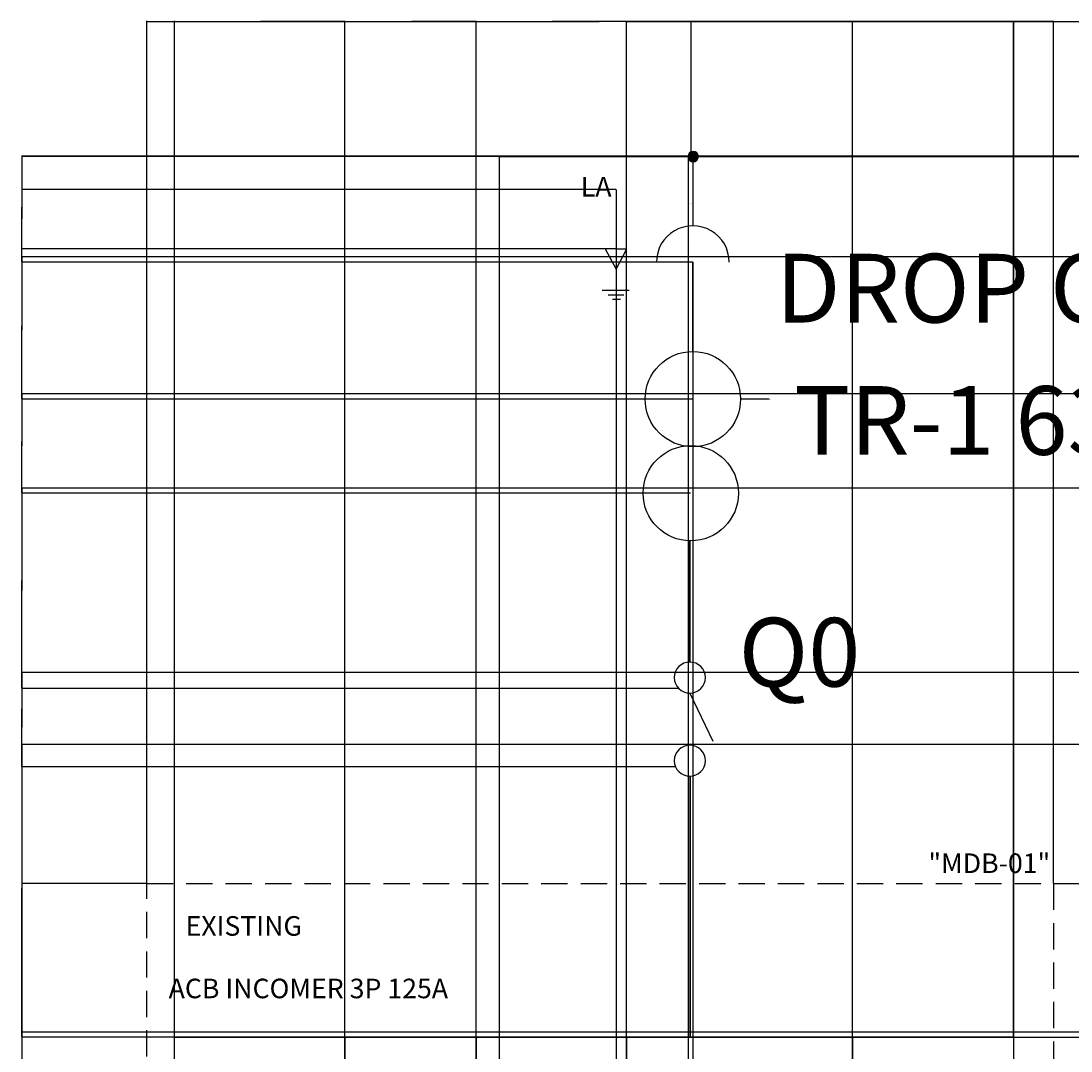
# Model space of a CAD drawing. Units: millimetres. Extents: x 1832 to 3146, y 927 to 1751.
# Tile 2 of 4: x 1832 to 2339, y 1253 to 1751. Entities that reach past the tile are written whole.
import ezdxf

# ---------------------------------------------------------------- set-up
doc = ezdxf.new("R2010")
doc.units = ezdxf.units.MM
doc.header["$MEASUREMENT"] = 0
doc.linetypes.add('DASHED', pattern=[19.05, 12.7, -6.35])
doc.layers.get('0').update_dxf_attribs({"color": 2, "lineweight": 35})
doc.layers.get('0').transparency = 0.01
for name, color, linetype, lineweight in [('A-ANNO-DIMS', 2, 'Continuous', 18), ('E-ANNO-TEXT', 7, 'Continuous', 18), ('E-POWR-EQPM', 2, 'Continuous', 25), ('E-POWR-PNLS', 3, 'DASHED', 25), ('E-POWR-WIRE', 7, 'Continuous', 35)]:
    doc.layers.add(name, color=color, linetype=linetype, lineweight=lineweight)
doc.styles.get("Standard").update_dxf_attribs({"font": 'arial.ttf'})
doc.dimstyles.get("Standard").update_dxf_attribs({"dimtxt": 0.18, "dimasz": 0.18, "dimexe": 0.18, "dimexo": 0.0625, "dimgap": 0.09, "dimtad": 0, "dimtih": 1, "dimtoh": 1, "dimdec": 4, "dimzin": 0, "dimdsep": 46, "dimtxsty": 'Standard', "dimcen": 0.09, "dimadec": 0, "dimazin": 0, "dimtfac": 1, "dimtdec": 4, "dimtofl": 0, "dimtmove": 0, "dimatfit": 3, "dimfxl": 1, "dimtolj": 1, "dimtzin": 0, "dimarcsym": 0})

# ---------------------------------------------------------------- blocks, each defined once
blk = doc.blocks.new('CB-INCOMER')
blk.add_line((2155.16, 1426.14), (2166.26, 1402.88))
for points in [[(2147.67, 1433.64, 1), (2162.67, 1433.64, 1)], [(2147.67, 1393.5, 1), (2162.67, 1393.5, 1)]]:
    blk.add_lwpolyline(points, format="xyb", close=True)
blk = doc.blocks.new('LIGHTNING-ARRESTER')
for p, q in [((2119.54, 1669.38), (2119.54, 1640.82)), ((2119.54, 1640.82), (2114.27, 1640.82)), ((2114.27, 1640.82), (2119.54, 1630.9)), ((2119.54, 1640.82), (2124.8, 1640.82)), ((2119.54, 1630.9), (2124.8, 1640.82)), ((2119.54, 1630.9), (2119.54, 1620.77)), ((2112.86, 1620.77), (2125.9, 1620.77)), ((2115.79, 1618.51), (2123.28, 1618.51)), ((2117.89, 1616.41), (2121.66, 1616.41))]:
    blk.add_line(p, q)
blk = doc.blocks.new('DROPOUT-FUSE')
h = blk.add_hatch(color=256)
h.dxf.hatch_style = 1
h.paths.add_polyline_path([(2154.3, 1685.32), (2159.3, 1685.32, 1)])
h.paths.add_polyline_path([(2159.3, 1685.32), (2154.3, 1685.32, 1)])
blk.add_line((2156.63, 1682.82), (2156.63, 1651.9))
blk.add_lwpolyline([(2154.3, 1685.32, 1), (2159.3, 1685.32, 1)], format="xyb", close=True)
blk.add_arc((2156.63, 1634.33), 17.57, 359.971, 180.029)
blk = doc.blocks.new('TRANSFORMER')
for centre in [(2156.63, 1568.17), (2155.63, 1522.72)]:
    blk.add_circle(centre, 23.01)
blk = doc.blocks.new('*D11')
at = {"layer": 'A-ANNO-DIMS', "color": 0, "lineweight": -2, "transparency": 16777216}
for p, q in [((1892.88, 1334.1), (1832.41, 1334.1)), ((1832.59, 1333.92), (1832.59, 1168.69)), ((1832.59, 1003.11), (1832.59, 1168.33)), ((1892.88, 1002.93), (1832.41, 1002.93))]:
    blk.add_line(p, q, dxfattribs=at)
at = {"layer": 'A-ANNO-DIMS', "color": 0, "lineweight": 35, "transparency": 16777216}
for points in [[(1832.56, 1333.92), (1832.62, 1333.92), (1832.59, 1334.1)], [(1832.56, 1003.11), (1832.62, 1003.11), (1832.59, 1002.93)]]:
    blk.add_solid(points, dxfattribs=at)
at = {"layer": 'Defpoints', "color": 0, "lineweight": 35, "transparency": 16777216}
for p in [(1832.59, 1334.1), (1892.94, 1334.1), (1892.94, 1002.93)]:
    blk.add_point(p, dxfattribs=at)
at = {"layer": 'A-ANNO-DIMS', "color": 0, "transparency": 16777216, "insert": (1832.59, 1168.51), "char_height": 0.18, "attachment_point": 5}
blk.add_mtext('\\A1;331.2', dxfattribs=at)
blk = doc.blocks.new('*D12')
at = {"layer": 'A-ANNO-DIMS', "color": 0, "lineweight": -2, "transparency": 16777216}
for p, q in [((1906.41, 1259.94), (1906.41, 1750.84)), ((1906.59, 1750.66), (1947.09, 1750.66)), ((1988.37, 1750.66), (1947.87, 1750.66)), ((1988.55, 1259.94), (1988.55, 1750.84))]:
    blk.add_line(p, q, dxfattribs=at)
at = {"layer": 'A-ANNO-DIMS', "color": 0, "lineweight": 35, "transparency": 16777216}
for points in [[(1906.59, 1750.69), (1906.59, 1750.63), (1906.41, 1750.66)], [(1988.37, 1750.69), (1988.37, 1750.63), (1988.55, 1750.66)]]:
    blk.add_solid(points, dxfattribs=at)
at = {"layer": 'Defpoints', "color": 0, "lineweight": 35, "transparency": 16777216}
for p in [(1988.55, 1750.66), (1906.41, 1259.88), (1988.55, 1259.88)]:
    blk.add_point(p, dxfattribs=at)
at = {"layer": 'A-ANNO-DIMS', "color": 0, "transparency": 16777216, "insert": (1947.48, 1750.66), "char_height": 0.18, "attachment_point": 5}
blk.add_mtext('\\A1;82.14', dxfattribs=at)
blk = doc.blocks.new('*D13')
at = {"layer": 'A-ANNO-DIMS', "color": 0, "lineweight": -2, "transparency": 16777216}
for p, q in [((1988.55, 1259.94), (1988.55, 1750.84)), ((1988.73, 1750.66), (2019.92, 1750.66)), ((2051.9, 1750.66), (2020.71, 1750.66)), ((2052.08, 1259.94), (2052.08, 1750.84))]:
    blk.add_line(p, q, dxfattribs=at)
at = {"layer": 'A-ANNO-DIMS', "color": 0, "lineweight": 35, "transparency": 16777216}
for points in [[(1988.73, 1750.69), (1988.73, 1750.63), (1988.55, 1750.66)], [(2051.9, 1750.69), (2051.9, 1750.63), (2052.08, 1750.66)]]:
    blk.add_solid(points, dxfattribs=at)
at = {"layer": 'Defpoints', "color": 0, "lineweight": 35, "transparency": 16777216}
for p in [(2052.08, 1750.66), (1988.55, 1259.88), (2052.08, 1259.88)]:
    blk.add_point(p, dxfattribs=at)
at = {"layer": 'A-ANNO-DIMS', "color": 0, "transparency": 16777216, "insert": (2020.31, 1750.66), "char_height": 0.18, "attachment_point": 5}
blk.add_mtext('\\A1;63.53', dxfattribs=at)
blk = doc.blocks.new('*D14')
at = {"layer": 'A-ANNO-DIMS', "color": 0, "lineweight": -2, "transparency": 16777216}
for p, q in [((2052.08, 1259.94), (2052.08, 1750.84)), ((2052.26, 1750.66), (2087.91, 1750.66)), ((2124.35, 1750.66), (2088.7, 1750.66)), ((2124.53, 1259.94), (2124.53, 1750.84))]:
    blk.add_line(p, q, dxfattribs=at)
at = {"layer": 'A-ANNO-DIMS', "color": 0, "lineweight": 35, "transparency": 16777216}
for points in [[(2052.26, 1750.69), (2052.26, 1750.63), (2052.08, 1750.66)], [(2124.35, 1750.69), (2124.35, 1750.63), (2124.53, 1750.66)]]:
    blk.add_solid(points, dxfattribs=at)
at = {"layer": 'Defpoints', "color": 0, "lineweight": 35, "transparency": 16777216}
for p in [(2124.53, 1750.66), (2052.08, 1259.88), (2124.53, 1259.88)]:
    blk.add_point(p, dxfattribs=at)
at = {"layer": 'A-ANNO-DIMS', "color": 0, "transparency": 16777216, "insert": (2088.31, 1750.66), "char_height": 0.18, "attachment_point": 5}
blk.add_mtext('\\A1;72.45', dxfattribs=at)
blk = doc.blocks.new('*D15')
at = {"layer": 'A-ANNO-DIMS', "color": 0, "lineweight": -2, "transparency": 16777216}
for p, q in [((2124.53, 1259.94), (2124.53, 1750.84)), ((2124.71, 1750.66), (2178.71, 1750.66)), ((2233.62, 1750.66), (2179.62, 1750.66)), ((2233.8, 1259.94), (2233.8, 1750.84))]:
    blk.add_line(p, q, dxfattribs=at)
at = {"layer": 'A-ANNO-DIMS', "color": 0, "lineweight": 35, "transparency": 16777216}
for points in [[(2124.71, 1750.69), (2124.71, 1750.63), (2124.53, 1750.66)], [(2233.62, 1750.69), (2233.62, 1750.63), (2233.8, 1750.66)]]:
    blk.add_solid(points, dxfattribs=at)
at = {"layer": 'Defpoints', "color": 0, "lineweight": 35, "transparency": 16777216}
for p in [(2233.8, 1750.66), (2124.53, 1259.88), (2233.8, 1259.88)]:
    blk.add_point(p, dxfattribs=at)
at = {"layer": 'A-ANNO-DIMS', "color": 0, "transparency": 16777216, "insert": (2179.17, 1750.66), "char_height": 0.18, "attachment_point": 5}
blk.add_mtext('\\A1;109.27', dxfattribs=at)
blk = doc.blocks.new('*D21')
at = {"layer": 'A-ANNO-DIMS', "color": 0, "lineweight": -2, "transparency": 16777216}
for p, q in [((2155.83, 1687.68), (2155.83, 1750.84)), ((2156.01, 1750.66), (2407.13, 1750.66)), ((2659.03, 1750.66), (2407.91, 1750.66)), ((2659.21, 1690.18), (2659.21, 1750.84))]:
    blk.add_line(p, q, dxfattribs=at)
at = {"layer": 'A-ANNO-DIMS', "color": 0, "lineweight": 35, "transparency": 16777216}
for points in [[(2156.01, 1750.69), (2156.01, 1750.63), (2155.83, 1750.66)], [(2659.03, 1750.69), (2659.03, 1750.63), (2659.21, 1750.66)]]:
    blk.add_solid(points, dxfattribs=at)
at = {"layer": 'Defpoints', "color": 0, "lineweight": 35, "transparency": 16777216}
for p in [(2659.21, 1750.66), (2659.21, 1690.11), (2155.83, 1687.62)]:
    blk.add_point(p, dxfattribs=at)
at = {"layer": 'A-ANNO-DIMS', "color": 0, "transparency": 16777216, "insert": (2407.52, 1750.66), "char_height": 0.18, "attachment_point": 5}
blk.add_mtext('\\A1;503.4', dxfattribs=at)
blk = doc.blocks.new('*D23')
at = {"layer": 'A-ANNO-DIMS', "color": 0, "lineweight": -2, "transparency": 16777216}
for p, q in [((2156.54, 1568.17), (2156.72, 1568.17)), ((2156.63, 1568.08), (2156.63, 1568.26)), ((2193.45, 1568.17), (2179.82, 1568.17))]:
    blk.add_line(p, q, dxfattribs=at)
at = {"layer": 'A-ANNO-DIMS', "color": 0, "lineweight": 35, "transparency": 16777216}
blk.add_solid([(2179.82, 1568.2), (2179.82, 1568.14), (2179.64, 1568.17)], dxfattribs=at)
at = {"layer": 'Defpoints', "color": 0, "lineweight": 35, "transparency": 16777216}
for p in [(2133.62, 1568.17), (2179.64, 1568.17)]:
    blk.add_point(p, dxfattribs=at)
at = {"layer": 'A-ANNO-DIMS', "color": 0, "transparency": 16777216, "insert": (2194.13, 1568.17), "char_height": 0.18, "attachment_point": 5}
blk.add_mtext('\\A1;4X ∅46.02', dxfattribs=at)
blk = doc.blocks.new('*D24')
at = {"layer": 'A-ANNO-DIMS', "color": 0, "lineweight": -2, "transparency": 16777216}
for p, q in [((2156.45, 1662.44), (2156.63, 1662.44)), ((2156.63, 1662.44), (2156.63, 1652.08)), ((2156.54, 1634.33), (2156.72, 1634.33)), ((2156.63, 1634.24), (2156.63, 1634.42))]:
    blk.add_line(p, q, dxfattribs=at)
at = {"layer": 'A-ANNO-DIMS', "color": 0, "lineweight": 35, "transparency": 16777216}
blk.add_solid([(2156.66, 1652.08), (2156.6, 1652.08), (2156.63, 1651.9)], dxfattribs=at)
at = {"layer": 'Defpoints', "color": 0, "lineweight": 35, "transparency": 16777216}
for p in [(2156.63, 1651.9), (2156.63, 1634.33)]:
    blk.add_point(p, dxfattribs=at)
at = {"layer": 'A-ANNO-DIMS', "color": 0, "transparency": 16777216, "insert": (2155.71, 1662.44), "char_height": 0.18, "attachment_point": 5}
blk.add_mtext('\\A1;2X R17.565', dxfattribs=at)
blk = doc.blocks.new('*D25')
at = {"layer": 'A-ANNO-DIMS', "color": 0, "lineweight": -2, "transparency": 16777216}
for p, q in [((1892.94, 1334.16), (1892.94, 1750.84)), ((1893.12, 1750.66), (2111.37, 1750.66)), ((2330.55, 1750.66), (2112.3, 1750.66)), ((2330.73, 1334.16), (2330.73, 1750.84))]:
    blk.add_line(p, q, dxfattribs=at)
at = {"layer": 'A-ANNO-DIMS', "color": 0, "lineweight": 35, "transparency": 16777216}
for points in [[(1893.12, 1750.69), (1893.12, 1750.63), (1892.94, 1750.66)], [(2330.55, 1750.69), (2330.55, 1750.63), (2330.73, 1750.66)]]:
    blk.add_solid(points, dxfattribs=at)
at = {"layer": 'Defpoints', "color": 0, "lineweight": 35, "transparency": 16777216}
for p in [(2330.73, 1750.66), (1892.94, 1334.1), (2330.73, 1334.1)]:
    blk.add_point(p, dxfattribs=at)
at = {"layer": 'A-ANNO-DIMS', "color": 0, "transparency": 16777216, "insert": (2111.83, 1750.66), "char_height": 0.18, "attachment_point": 5}
blk.add_mtext('\\A1;437.79', dxfattribs=at)
blk = doc.blocks.new('*D27')
at = {"layer": 'A-ANNO-DIMS', "color": 0, "lineweight": -2, "transparency": 16777216}
for p, q in [((1906.41, 1015.38), (1906.41, 1750.84)), ((1906.59, 1750.66), (2108.57, 1750.66)), ((2311.47, 1750.66), (2109.5, 1750.66)), ((2311.65, 1015.38), (2311.65, 1750.84))]:
    blk.add_line(p, q, dxfattribs=at)
at = {"layer": 'A-ANNO-DIMS', "color": 0, "lineweight": 35, "transparency": 16777216}
for points in [[(1906.59, 1750.69), (1906.59, 1750.63), (1906.41, 1750.66)], [(2311.47, 1750.69), (2311.47, 1750.63), (2311.65, 1750.66)]]:
    blk.add_solid(points, dxfattribs=at)
at = {"layer": 'Defpoints', "color": 0, "lineweight": 35, "transparency": 16777216}
for p in [(2311.65, 1750.66), (1906.41, 1015.32), (2311.65, 1015.32)]:
    blk.add_point(p, dxfattribs=at)
at = {"layer": 'A-ANNO-DIMS', "color": 0, "transparency": 16777216, "insert": (2109.03, 1750.66), "char_height": 0.18, "attachment_point": 5}
blk.add_mtext('\\A1;405.24', dxfattribs=at)
blk = doc.blocks.new('*D29')
at = {"layer": 'A-ANNO-DIMS', "color": 0, "lineweight": -2, "transparency": 16777216}
for p, q in [((2233.8, 1259.94), (2233.8, 1750.84)), ((2233.98, 1750.66), (2272.23, 1750.66)), ((2311.23, 1750.66), (2272.98, 1750.66)), ((2311.41, 1259.94), (2311.41, 1750.84))]:
    blk.add_line(p, q, dxfattribs=at)
at = {"layer": 'A-ANNO-DIMS', "color": 0, "lineweight": 35, "transparency": 16777216}
for points in [[(2233.98, 1750.69), (2233.98, 1750.63), (2233.8, 1750.66)], [(2311.23, 1750.69), (2311.23, 1750.63), (2311.41, 1750.66)]]:
    blk.add_solid(points, dxfattribs=at)
at = {"layer": 'Defpoints', "color": 0, "lineweight": 35, "transparency": 16777216}
for p in [(2311.41, 1750.66), (2233.8, 1259.88), (2311.41, 1259.88)]:
    blk.add_point(p, dxfattribs=at)
at = {"layer": 'A-ANNO-DIMS', "color": 0, "transparency": 16777216, "insert": (2272.61, 1750.66), "char_height": 0.18, "attachment_point": 5}
blk.add_mtext('\\A1;77.61', dxfattribs=at)
blk = doc.blocks.new('*D32')
at = {"layer": 'A-ANNO-DIMS', "color": 0, "lineweight": -2, "transparency": 16777216}
for p, q in [((2063.17, 1685.25), (2063.17, 927.26)), ((2154.3, 1685.25), (2154.3, 927.26)), ((2063.35, 927.44), (2108.34, 927.44)), ((2154.12, 927.44), (2109.13, 927.44))]:
    blk.add_line(p, q, dxfattribs=at)
at = {"layer": 'A-ANNO-DIMS', "color": 0, "lineweight": 35, "transparency": 16777216}
for points in [[(2063.35, 927.47), (2063.35, 927.41), (2063.17, 927.44)], [(2154.12, 927.47), (2154.12, 927.41), (2154.3, 927.44)]]:
    blk.add_solid(points, dxfattribs=at)
at = {"layer": 'Defpoints', "color": 0, "lineweight": 35, "transparency": 16777216}
for p in [(2063.17, 1685.32), (2154.3, 1685.32), (2154.3, 927.44)]:
    blk.add_point(p, dxfattribs=at)
at = {"layer": 'A-ANNO-DIMS', "color": 0, "transparency": 16777216, "insert": (2108.74, 927.44), "char_height": 0.18, "attachment_point": 5}
blk.add_mtext('\\A1;91.13', dxfattribs=at)
blk = doc.blocks.new('*D34')
at = {"layer": 'A-ANNO-DIMS', "color": 0, "lineweight": -2, "transparency": 16777216}
for p, q in [((2119.54, 1640.76), (2119.54, 927.26)), ((2156.63, 1634.27), (2156.63, 927.26)), ((2119.72, 927.44), (2137.69, 927.44)), ((2156.45, 927.44), (2138.48, 927.44))]:
    blk.add_line(p, q, dxfattribs=at)
at = {"layer": 'A-ANNO-DIMS', "color": 0, "lineweight": 35, "transparency": 16777216}
for points in [[(2119.72, 927.47), (2119.72, 927.41), (2119.54, 927.44)], [(2156.45, 927.47), (2156.45, 927.41), (2156.63, 927.44)]]:
    blk.add_solid(points, dxfattribs=at)
at = {"layer": 'Defpoints', "color": 0, "lineweight": 35, "transparency": 16777216}
for p in [(2119.54, 1640.82), (2156.63, 1634.33), (2156.63, 927.44)]:
    blk.add_point(p, dxfattribs=at)
at = {"layer": 'A-ANNO-DIMS', "color": 0, "transparency": 16777216, "insert": (2138.08, 927.44), "char_height": 0.18, "attachment_point": 5}
blk.add_mtext('\\A1;37.10', dxfattribs=at)
blk = doc.blocks.new('*D35')
at = {"layer": 'A-ANNO-DIMS', "color": 0, "lineweight": -2, "transparency": 16777216}
for p, q in [((2148.2, 1390.58), (1832.41, 1390.58)), ((1832.59, 1390.4), (1832.59, 1325.41)), ((1832.59, 1260.06), (1832.59, 1325.05)), ((2155.33, 1259.88), (1832.41, 1259.88))]:
    blk.add_line(p, q, dxfattribs=at)
at = {"layer": 'A-ANNO-DIMS', "color": 0, "lineweight": 35, "transparency": 16777216}
for points in [[(1832.56, 1390.4), (1832.62, 1390.4), (1832.59, 1390.58)], [(1832.56, 1260.06), (1832.62, 1260.06), (1832.59, 1259.88)]]:
    blk.add_solid(points, dxfattribs=at)
at = {"layer": 'Defpoints', "color": 0, "lineweight": 35, "transparency": 16777216}
for p in [(1832.59, 1390.58), (2148.26, 1390.58), (2155.39, 1259.88)]:
    blk.add_point(p, dxfattribs=at)
at = {"layer": 'A-ANNO-DIMS', "color": 0, "transparency": 16777216, "insert": (1832.59, 1325.23), "char_height": 0.18, "attachment_point": 5}
blk.add_mtext('\\A1;130.70', dxfattribs=at)
blk = doc.blocks.new('*D36')
at = {"layer": 'A-ANNO-DIMS', "color": 0, "lineweight": -2, "transparency": 16777216}
for p, q in [((2149.8, 1428.33), (1832.41, 1428.33)), ((1832.59, 1428.15), (1832.59, 1409.64)), ((1832.59, 1390.76), (1832.59, 1409.27)), ((2148.2, 1390.58), (1832.41, 1390.58))]:
    blk.add_line(p, q, dxfattribs=at)
at = {"layer": 'A-ANNO-DIMS', "color": 0, "lineweight": 35, "transparency": 16777216}
for points in [[(1832.56, 1428.15), (1832.62, 1428.15), (1832.59, 1428.33)], [(1832.56, 1390.76), (1832.62, 1390.76), (1832.59, 1390.58)]]:
    blk.add_solid(points, dxfattribs=at)
at = {"layer": 'Defpoints', "color": 0, "lineweight": 35, "transparency": 16777216}
for p in [(1832.59, 1428.33), (2149.87, 1428.33), (2148.26, 1390.58)]:
    blk.add_point(p, dxfattribs=at)
at = {"layer": 'A-ANNO-DIMS', "color": 0, "transparency": 16777216, "insert": (1832.59, 1409.46), "char_height": 0.18, "attachment_point": 5}
blk.add_mtext('\\A1;37.75', dxfattribs=at)
blk = doc.blocks.new('*D37')
at = {"layer": 'A-ANNO-DIMS', "color": 0, "lineweight": -2, "transparency": 16777216}
for p, q in [((2155.57, 1522.72), (1832.41, 1522.72)), ((1832.59, 1522.54), (1832.59, 1475.71)), ((1832.59, 1428.51), (1832.59, 1475.35)), ((2149.8, 1428.33), (1832.41, 1428.33))]:
    blk.add_line(p, q, dxfattribs=at)
at = {"layer": 'A-ANNO-DIMS', "color": 0, "lineweight": 35, "transparency": 16777216}
for points in [[(1832.56, 1522.54), (1832.62, 1522.54), (1832.59, 1522.72)], [(1832.56, 1428.51), (1832.62, 1428.51), (1832.59, 1428.33)]]:
    blk.add_solid(points, dxfattribs=at)
at = {"layer": 'Defpoints', "color": 0, "lineweight": 35, "transparency": 16777216}
for p in [(1832.59, 1522.72), (2155.63, 1522.72), (2149.87, 1428.33)]:
    blk.add_point(p, dxfattribs=at)
at = {"layer": 'A-ANNO-DIMS', "color": 0, "transparency": 16777216, "insert": (1832.59, 1475.53), "char_height": 0.18, "attachment_point": 5}
blk.add_mtext('\\A1;94.39', dxfattribs=at)
blk = doc.blocks.new('*D38')
at = {"layer": 'A-ANNO-DIMS', "color": 0, "lineweight": -2, "transparency": 16777216}
for p, q in [((2156.57, 1568.17), (1832.41, 1568.17)), ((1832.59, 1567.99), (1832.59, 1545.63)), ((1832.59, 1522.9), (1832.59, 1545.27)), ((2155.57, 1522.72), (1832.41, 1522.72))]:
    blk.add_line(p, q, dxfattribs=at)
at = {"layer": 'A-ANNO-DIMS', "color": 0, "lineweight": 35, "transparency": 16777216}
for points in [[(1832.56, 1567.99), (1832.62, 1567.99), (1832.59, 1568.17)], [(1832.56, 1522.9), (1832.62, 1522.9), (1832.59, 1522.72)]]:
    blk.add_solid(points, dxfattribs=at)
at = {"layer": 'Defpoints', "color": 0, "lineweight": 35, "transparency": 16777216}
for p in [(1832.59, 1568.17), (2156.63, 1568.17), (2155.63, 1522.72)]:
    blk.add_point(p, dxfattribs=at)
at = {"layer": 'A-ANNO-DIMS', "color": 0, "transparency": 16777216, "insert": (1832.59, 1545.45), "char_height": 0.18, "attachment_point": 5}
blk.add_mtext('\\A1;45.45', dxfattribs=at)
blk = doc.blocks.new('*D39')
at = {"layer": 'A-ANNO-DIMS', "color": 0, "lineweight": -2, "transparency": 16777216}
for p, q in [((2156.57, 1634.33), (1832.41, 1634.33)), ((1832.59, 1634.15), (1832.59, 1601.43)), ((1832.59, 1568.35), (1832.59, 1601.07)), ((2156.57, 1568.17), (1832.41, 1568.17))]:
    blk.add_line(p, q, dxfattribs=at)
at = {"layer": 'A-ANNO-DIMS', "color": 0, "lineweight": 35, "transparency": 16777216}
for points in [[(1832.56, 1634.15), (1832.62, 1634.15), (1832.59, 1634.33)], [(1832.56, 1568.35), (1832.62, 1568.35), (1832.59, 1568.17)]]:
    blk.add_solid(points, dxfattribs=at)
at = {"layer": 'Defpoints', "color": 0, "lineweight": 35, "transparency": 16777216}
for p in [(1832.59, 1634.33), (2156.63, 1634.33), (2156.63, 1568.17)]:
    blk.add_point(p, dxfattribs=at)
at = {"layer": 'A-ANNO-DIMS', "color": 0, "transparency": 16777216, "insert": (1832.59, 1601.25), "char_height": 0.18, "attachment_point": 5}
blk.add_mtext('\\A1;66.16', dxfattribs=at)
blk = doc.blocks.new('*D40')
at = {"layer": 'A-ANNO-DIMS', "color": 0, "lineweight": -2, "transparency": 16777216}
for p, q in [((2154.24, 1685.32), (1832.41, 1685.32)), ((1832.59, 1685.14), (1832.59, 1660.01)), ((1832.59, 1634.51), (1832.59, 1659.64)), ((2156.57, 1634.33), (1832.41, 1634.33))]:
    blk.add_line(p, q, dxfattribs=at)
at = {"layer": 'A-ANNO-DIMS', "color": 0, "lineweight": 35, "transparency": 16777216}
for points in [[(1832.56, 1685.14), (1832.62, 1685.14), (1832.59, 1685.32)], [(1832.56, 1634.51), (1832.62, 1634.51), (1832.59, 1634.33)]]:
    blk.add_solid(points, dxfattribs=at)
at = {"layer": 'Defpoints', "color": 0, "lineweight": 35, "transparency": 16777216}
for p in [(1832.59, 1685.32), (2154.3, 1685.32), (2156.63, 1634.33)]:
    blk.add_point(p, dxfattribs=at)
at = {"layer": 'A-ANNO-DIMS', "color": 0, "transparency": 16777216, "insert": (1832.59, 1659.82), "char_height": 0.18, "attachment_point": 5}
blk.add_mtext('\\A1;50.99', dxfattribs=at)
blk = doc.blocks.new('*D41')
at = {"layer": 'A-ANNO-DIMS', "color": 0, "lineweight": -2, "transparency": 16777216}
for p, q in [((2119.47, 1669.38), (1832.41, 1669.38)), ((1832.59, 1669.2), (1832.59, 1655.28)), ((1832.59, 1641), (1832.59, 1654.92)), ((2119.47, 1640.82), (1832.41, 1640.82))]:
    blk.add_line(p, q, dxfattribs=at)
at = {"layer": 'A-ANNO-DIMS', "color": 0, "lineweight": 35, "transparency": 16777216}
for points in [[(1832.56, 1669.2), (1832.62, 1669.2), (1832.59, 1669.38)], [(1832.56, 1641), (1832.62, 1641), (1832.59, 1640.82)]]:
    blk.add_solid(points, dxfattribs=at)
at = {"layer": 'Defpoints', "color": 0, "lineweight": 35, "transparency": 16777216}
for p in [(1832.59, 1669.38), (2119.54, 1669.38), (2119.54, 1640.82)]:
    blk.add_point(p, dxfattribs=at)
at = {"layer": 'A-ANNO-DIMS', "color": 0, "transparency": 16777216, "insert": (1832.59, 1655.1), "char_height": 0.18, "attachment_point": 5}
blk.add_mtext('\\A1;28.56', dxfattribs=at)
blk = doc.blocks.new('*D42')
at = {"layer": 'A-ANNO-DIMS', "color": 0, "lineweight": -2, "transparency": 16777216}
for p, q in [((1988.49, 1259.88), (1832.41, 1259.88)), ((1832.59, 1259.7), (1832.59, 1225.24)), ((1832.59, 1190.42), (1832.59, 1224.88)), ((1988.49, 1190.24), (1832.41, 1190.24))]:
    blk.add_line(p, q, dxfattribs=at)
at = {"layer": 'A-ANNO-DIMS', "color": 0, "lineweight": 35, "transparency": 16777216}
for points in [[(1832.56, 1259.7), (1832.62, 1259.7), (1832.59, 1259.88)], [(1832.56, 1190.42), (1832.62, 1190.42), (1832.59, 1190.24)]]:
    blk.add_solid(points, dxfattribs=at)
at = {"layer": 'Defpoints', "color": 0, "lineweight": 35, "transparency": 16777216}
for p in [(1988.55, 1259.88), (1832.59, 1190.24), (1988.55, 1190.24)]:
    blk.add_point(p, dxfattribs=at)
at = {"layer": 'A-ANNO-DIMS', "color": 0, "transparency": 16777216, "insert": (1832.59, 1225.06), "char_height": 0.18, "attachment_point": 5}
blk.add_mtext('\\A1;69.64', dxfattribs=at)
blk = doc.blocks.new('*D47')
at = {"layer": 'A-ANNO-DIMS', "color": 0, "lineweight": -2, "transparency": 16777216}
for p, q in [((2330.79, 1334.1), (3145.86, 1334.1)), ((3145.68, 1333.92), (3145.68, 1297.17)), ((3145.68, 1260.06), (3145.68, 1296.81)), ((2311.47, 1259.88), (3145.86, 1259.88))]:
    blk.add_line(p, q, dxfattribs=at)
at = {"layer": 'A-ANNO-DIMS', "color": 0, "lineweight": 35, "transparency": 16777216}
for points in [[(3145.65, 1333.92), (3145.71, 1333.92), (3145.68, 1334.1)], [(3145.65, 1260.06), (3145.71, 1260.06), (3145.68, 1259.88)]]:
    blk.add_solid(points, dxfattribs=at)
at = {"layer": 'Defpoints', "color": 0, "lineweight": 35, "transparency": 16777216}
for p in [(2330.73, 1334.1), (2311.41, 1259.88), (3145.68, 1259.88)]:
    blk.add_point(p, dxfattribs=at)
at = {"layer": 'A-ANNO-DIMS', "color": 0, "transparency": 16777216, "insert": (3145.68, 1296.99), "char_height": 0.18, "attachment_point": 5}
blk.add_mtext('\\A1;74.22', dxfattribs=at)
blk = doc.blocks.new('*D50')
at = {"layer": 'A-ANNO-DIMS', "color": 0, "lineweight": -2, "transparency": 16777216}
for p, q in [((2663.8, 1401.3), (1832.41, 1401.3)), ((1832.59, 1401.12), (1832.59, 1332.02)), ((1832.59, 1262.55), (1832.59, 1331.65)), ((2658.71, 1262.37), (1832.41, 1262.37))]:
    blk.add_line(p, q, dxfattribs=at)
at = {"layer": 'A-ANNO-DIMS', "color": 0, "lineweight": 35, "transparency": 16777216}
for points in [[(1832.56, 1401.12), (1832.62, 1401.12), (1832.59, 1401.3)], [(1832.56, 1262.55), (1832.62, 1262.55), (1832.59, 1262.37)]]:
    blk.add_solid(points, dxfattribs=at)
at = {"layer": 'Defpoints', "color": 0, "lineweight": 35, "transparency": 16777216}
for p in [(1832.59, 1401.3), (2663.86, 1401.3), (2658.78, 1262.37)]:
    blk.add_point(p, dxfattribs=at)
at = {"layer": 'A-ANNO-DIMS', "color": 0, "transparency": 16777216, "insert": (1832.59, 1331.83), "char_height": 0.18, "attachment_point": 5}
blk.add_mtext('\\A1;138.92', dxfattribs=at)
blk = doc.blocks.new('*D51')
at = {"layer": 'A-ANNO-DIMS', "color": 0, "lineweight": -2, "transparency": 16777216}
for p, q in [((2665.99, 1436.13), (1832.41, 1436.13)), ((1832.59, 1435.95), (1832.59, 1418.9)), ((1832.59, 1401.48), (1832.59, 1418.53)), ((2663.8, 1401.3), (1832.41, 1401.3))]:
    blk.add_line(p, q, dxfattribs=at)
at = {"layer": 'A-ANNO-DIMS', "color": 0, "lineweight": 35, "transparency": 16777216}
for points in [[(1832.56, 1435.95), (1832.62, 1435.95), (1832.59, 1436.13)], [(1832.56, 1401.48), (1832.62, 1401.48), (1832.59, 1401.3)]]:
    blk.add_solid(points, dxfattribs=at)
at = {"layer": 'Defpoints', "color": 0, "lineweight": 35, "transparency": 16777216}
for p in [(1832.59, 1436.13), (2666.06, 1436.13), (2663.86, 1401.3)]:
    blk.add_point(p, dxfattribs=at)
at = {"layer": 'A-ANNO-DIMS', "color": 0, "transparency": 16777216, "insert": (1832.59, 1418.71), "char_height": 0.18, "attachment_point": 5}
blk.add_mtext('\\A1;34.83', dxfattribs=at)
blk = doc.blocks.new('*D52')
at = {"layer": 'A-ANNO-DIMS', "color": 0, "lineweight": -2, "transparency": 16777216}
for p, q in [((2658.96, 1525.22), (1832.41, 1525.22)), ((1832.59, 1525.04), (1832.59, 1480.86)), ((1832.59, 1436.31), (1832.59, 1480.49)), ((2665.99, 1436.13), (1832.41, 1436.13))]:
    blk.add_line(p, q, dxfattribs=at)
at = {"layer": 'A-ANNO-DIMS', "color": 0, "lineweight": 35, "transparency": 16777216}
for points in [[(1832.56, 1525.04), (1832.62, 1525.04), (1832.59, 1525.22)], [(1832.56, 1436.31), (1832.62, 1436.31), (1832.59, 1436.13)]]:
    blk.add_solid(points, dxfattribs=at)
at = {"layer": 'Defpoints', "color": 0, "lineweight": 35, "transparency": 16777216}
for p in [(1832.59, 1525.22), (2659.02, 1525.22), (2666.06, 1436.13)]:
    blk.add_point(p, dxfattribs=at)
at = {"layer": 'A-ANNO-DIMS', "color": 0, "transparency": 16777216, "insert": (1832.59, 1480.67), "char_height": 0.18, "attachment_point": 5}
blk.add_mtext('\\A1;89.09', dxfattribs=at)
blk = doc.blocks.new('*D53')
at = {"layer": 'A-ANNO-DIMS', "color": 0, "lineweight": -2, "transparency": 16777216}
for p, q in [((2659.96, 1570.67), (1832.41, 1570.67)), ((1832.59, 1570.49), (1832.59, 1548.12)), ((1832.59, 1525.4), (1832.59, 1547.76)), ((2658.96, 1525.22), (1832.41, 1525.22))]:
    blk.add_line(p, q, dxfattribs=at)
at = {"layer": 'A-ANNO-DIMS', "color": 0, "lineweight": 35, "transparency": 16777216}
for points in [[(1832.56, 1570.49), (1832.62, 1570.49), (1832.59, 1570.67)], [(1832.56, 1525.4), (1832.62, 1525.4), (1832.59, 1525.22)]]:
    blk.add_solid(points, dxfattribs=at)
at = {"layer": 'Defpoints', "color": 0, "lineweight": 35, "transparency": 16777216}
for p in [(1832.59, 1570.67), (2660.02, 1570.67), (2659.02, 1525.22)]:
    blk.add_point(p, dxfattribs=at)
at = {"layer": 'A-ANNO-DIMS', "color": 0, "transparency": 16777216, "insert": (1832.59, 1547.94), "char_height": 0.18, "attachment_point": 5}
blk.add_mtext('\\A1;45.45', dxfattribs=at)
blk = doc.blocks.new('*D54')
at = {"layer": 'A-ANNO-DIMS', "color": 0, "lineweight": -2, "transparency": 16777216}
for p, q in [((2659.96, 1636.83), (1832.41, 1636.83)), ((1832.59, 1636.65), (1832.59, 1603.93)), ((1832.59, 1570.85), (1832.59, 1603.56)), ((2659.96, 1570.67), (1832.41, 1570.67))]:
    blk.add_line(p, q, dxfattribs=at)
at = {"layer": 'A-ANNO-DIMS', "color": 0, "lineweight": 35, "transparency": 16777216}
for points in [[(1832.56, 1636.65), (1832.62, 1636.65), (1832.59, 1636.83)], [(1832.56, 1570.85), (1832.62, 1570.85), (1832.59, 1570.67)]]:
    blk.add_solid(points, dxfattribs=at)
at = {"layer": 'Defpoints', "color": 0, "lineweight": 35, "transparency": 16777216}
for p in [(1832.59, 1636.83), (2660.02, 1636.83), (2660.02, 1570.67)]:
    blk.add_point(p, dxfattribs=at)
at = {"layer": 'A-ANNO-DIMS', "color": 0, "transparency": 16777216, "insert": (1832.59, 1603.75), "char_height": 0.18, "attachment_point": 5}
blk.add_mtext('\\A1;66.16', dxfattribs=at)
blk = doc.blocks.new('*D55')
at = {"layer": 'A-ANNO-DIMS', "color": 0, "lineweight": -2, "transparency": 16777216}
for p, q in [((2659.15, 1685.51), (1832.41, 1685.51)), ((1832.59, 1685.33), (1832.59, 1661.35)), ((1832.59, 1637.01), (1832.59, 1660.98)), ((2659.96, 1636.83), (1832.41, 1636.83))]:
    blk.add_line(p, q, dxfattribs=at)
at = {"layer": 'A-ANNO-DIMS', "color": 0, "lineweight": 35, "transparency": 16777216}
for points in [[(1832.56, 1685.33), (1832.62, 1685.33), (1832.59, 1685.51)], [(1832.56, 1637.01), (1832.62, 1637.01), (1832.59, 1636.83)]]:
    blk.add_solid(points, dxfattribs=at)
at = {"layer": 'Defpoints', "color": 0, "lineweight": 35, "transparency": 16777216}
for p in [(1832.59, 1685.51), (2659.21, 1685.51), (2660.02, 1636.83)]:
    blk.add_point(p, dxfattribs=at)
at = {"layer": 'A-ANNO-DIMS', "color": 0, "transparency": 16777216, "insert": (1832.59, 1661.17), "char_height": 0.18, "attachment_point": 5}
blk.add_mtext('\\A1;48.68', dxfattribs=at)
blk = doc.blocks.new('*D57')
at = {"layer": 'A-ANNO-DIMS', "color": 0, "lineweight": -2, "transparency": 16777216}
for p, q in [((2156.54, 1568.17), (2156.72, 1568.17)), ((2156.63, 1568.08), (2156.63, 1568.26)), ((2193.45, 1568.17), (2179.82, 1568.17))]:
    blk.add_line(p, q, dxfattribs=at)
at = {"layer": 'A-ANNO-DIMS', "color": 0, "lineweight": 35, "transparency": 16777216}
blk.add_solid([(2179.82, 1568.2), (2179.82, 1568.14), (2179.64, 1568.17)], dxfattribs=at)
at = {"layer": 'Defpoints', "color": 0, "lineweight": 35, "transparency": 16777216}
for p in [(2133.62, 1568.17), (2179.64, 1568.17)]:
    blk.add_point(p, dxfattribs=at)
at = {"layer": 'A-ANNO-DIMS', "color": 0, "transparency": 16777216, "insert": (2194.13, 1568.17), "char_height": 0.18, "attachment_point": 5}
blk.add_mtext('\\A1;4X ∅46.02', dxfattribs=at)
blk = doc.blocks.new('*D58')
at = {"layer": 'A-ANNO-DIMS', "color": 0, "lineweight": -2, "transparency": 16777216}
for p, q in [((2156.45, 1662.44), (2156.63, 1662.44)), ((2156.63, 1662.44), (2156.63, 1652.08)), ((2156.54, 1634.33), (2156.72, 1634.33)), ((2156.63, 1634.24), (2156.63, 1634.42))]:
    blk.add_line(p, q, dxfattribs=at)
at = {"layer": 'A-ANNO-DIMS', "color": 0, "lineweight": 35, "transparency": 16777216}
blk.add_solid([(2156.66, 1652.08), (2156.6, 1652.08), (2156.63, 1651.9)], dxfattribs=at)
at = {"layer": 'Defpoints', "color": 0, "lineweight": 35, "transparency": 16777216}
for p in [(2156.63, 1651.9), (2156.63, 1634.33)]:
    blk.add_point(p, dxfattribs=at)
at = {"layer": 'A-ANNO-DIMS', "color": 0, "transparency": 16777216, "insert": (2155.71, 1662.44), "char_height": 0.18, "attachment_point": 5}
blk.add_mtext('\\A1;2X R17.565', dxfattribs=at)

msp = doc.modelspace()

# ---------------------------------------------------------------- linework, layer by layer
at = {"layer": 'E-POWR-PNLS'}
msp.add_lwpolyline([(1892.9387, 1334.0963), (2330.7306, 1334.0963), (2330.7306, 1002.9254), (1892.9387, 1002.9254)], close=True, dxfattribs=at)
at = {"layer": 'E-POWR-WIRE'}
for p, q in [((2063.171, 1685.3164), (2684.8145, 1685.3164)), ((2156.6335, 1634.3311), (2156.6335, 1591.1811)), ((2155.1688, 1499.7184), (2155.1688, 1441.136)), ((2155.3893, 1386.0027), (2155.3893, 1259.8778)), ((1906.4128, 1259.8778), (2311.4119, 1259.8778)), ((1988.5483, 1259.8778), (1988.5483, 1190.2428)), ((2052.0805, 1259.8778), (2052.0805, 1190.2428)), ((2124.5321, 1259.8778), (2124.5321, 1190.2428)), ((2233.8033, 1259.8778), (2233.8033, 1190.2428))]:
    msp.add_line(p, q, dxfattribs=at)

# ---------------------------------------------------------------- block references
at = {"layer": 'E-POWR-EQPM'}
for name in ['DROPOUT-FUSE', 'LIGHTNING-ARRESTER', 'TRANSFORMER', 'CB-INCOMER']:
    msp.add_blockref(name, (0, 0), dxfattribs=at)

# ---------------------------------------------------------------- texts
at = {"layer": 'E-ANNO-TEXT'}
for s, height, p in [('LA', 9.44797, (2102.5304, 1666.0507)), ('DROP OUT FUSE', 33.205653, (2196.7504, 1605.1502)), ('TR-1 630 KVA', 33.205653, (2205.5164, 1541.2551)), ('Q0', 33.20565, (2178.771, 1429.277)), ('"MDB-01"', 9.44797, (2270.3965, 1339.2404)), ('EXISTING', 9.44797, (1911.6923, 1308.9419)), ('ACB INCOMER 3P 125A', 9.447971, (1903.5021, 1278.734))]:
    msp.add_text(s, height=height, dxfattribs=at).set_placement(p)

# ---------------------------------------------------------------- dimensions: what is measured, and where the dimension line sits
at = {"layer": 'A-ANNO-DIMS'}
for base, p1, p2, override, picture, middle in [((2330.7306, 1750.6609), (1892.9387, 1334.0963), (2330.7306, 1334.0963), {"dimdec": 2, "dimlfac": 1, "dimrnd": 0, "dimzin": 0, "dimdsep": 46, "dimlunit": 2}, '*D25', (2111.8347, 1750.6609)), ((1988.5483, 1750.6609), (1906.4128, 1259.8778), (1988.5483, 1259.8778), {"dimdec": 2, "dimlfac": 1, "dimrnd": 0, "dimzin": 0, "dimdsep": 46, "dimlunit": 2}, '*D12', (1947.4805, 1750.6609)), ((2311.6539, 1750.6609), (1906.4128, 1015.321), (2311.6539, 1015.321), {"dimdec": 2, "dimlfac": 1, "dimrnd": 0, "dimzin": 0, "dimdsep": 46, "dimlunit": 2}, '*D27', (2109.0334, 1750.6609)), ((2052.0805, 1750.6609), (1988.5483, 1259.8778), (2052.0805, 1259.8778), {"dimdec": 2, "dimlfac": 1, "dimrnd": 0, "dimzin": 0, "dimdsep": 46, "dimlunit": 2}, '*D13', (2020.3144, 1750.6609)), ((2124.5321, 1750.6609), (2052.0805, 1259.8778), (2124.5321, 1259.8778), {"dimdec": 2, "dimlfac": 1, "dimrnd": 0, "dimzin": 0, "dimdsep": 46, "dimlunit": 2}, '*D14', (2088.3063, 1750.6609)), ((2233.8033, 1750.6609), (2124.5321, 1259.8778), (2233.8033, 1259.8778), {"dimdec": 2, "dimlfac": 1, "dimrnd": 0, "dimzin": 0, "dimdsep": 46, "dimlunit": 2}, '*D15', (2179.1677, 1750.6609)), ((2659.2142, 1750.6609), (2155.8261, 1687.62), (2659.2142, 1690.1145), {"dimdec": 1, "dimlfac": 1, "dimrnd": 0, "dimzin": 0, "dimdsep": 46, "dimlunit": 2}, '*D21', (2407.5202, 1750.6609)), ((2311.4119, 1750.6609), (2233.8033, 1259.8778), (2311.4119, 1259.8778), {"dimdec": 2, "dimlfac": 1, "dimrnd": 0, "dimzin": 0, "dimdsep": 46, "dimlunit": 2}, '*D29', (2272.6076, 1750.6609)), ((2154.2992, 927.4392), (2063.171, 1685.3164), (2154.2992, 1685.3164), {"dimdec": 2, "dimlfac": 1, "dimrnd": 0, "dimzin": 0, "dimdsep": 46, "dimlunit": 2}, '*D32', (2108.7351, 927.4392)), ((2156.6335, 927.4392), (2119.5362, 1640.8227), (2156.6335, 1634.3311), {"dimdec": 2, "dimlfac": 1, "dimrnd": 0, "dimzin": 0, "dimdsep": 46, "dimlunit": 2}, '*D34', (2138.0848, 927.4392))]:
    dim = msp.add_linear_dim(base=base, p1=p1, p2=p2, dimstyle='Standard', override=override, dxfattribs=at)
    dim.commit()
    dim.dimension.update_dxf_attribs({"geometry": picture, "text_midpoint": middle})
for base, p1, p2, override, picture, middle in [((1832.5887, 1685.5074), (2660.0216, 1636.8256), (2659.2142, 1685.5074), {"dimdec": 2, "dimlfac": 1, "dimrnd": 0, "dimzin": 0, "dimdsep": 46, "dimlunit": 2}, '*D55', (1832.5887, 1661.1665)), ((1832.5887, 1685.3164), (2156.6335, 1634.3311), (2154.2992, 1685.3164), {"dimdec": 2, "dimlfac": 1, "dimrnd": 0, "dimzin": 0, "dimdsep": 46, "dimlunit": 2}, '*D40', (1832.5887, 1659.8238)), ((1832.5887, 1669.3813), (2119.5362, 1640.8227), (2119.5362, 1669.3813), {"dimdec": 2, "dimlfac": 1, "dimrnd": 0, "dimzin": 0, "dimdsep": 46, "dimlunit": 2}, '*D41', (1832.5887, 1655.102)), ((1832.5887, 1636.8256), (2660.0216, 1570.6655), (2660.0216, 1636.8256), {"dimdec": 2, "dimlfac": 1, "dimrnd": 0, "dimzin": 0, "dimdsep": 46, "dimlunit": 2}, '*D54', (1832.5887, 1603.7456)), ((1832.5887, 1634.3311), (2156.6335, 1568.171), (2156.6335, 1634.3311), {"dimdec": 2, "dimlfac": 1, "dimrnd": 0, "dimzin": 0, "dimdsep": 46, "dimlunit": 2}, '*D39', (1832.5887, 1601.2511)), ((1832.5887, 1570.6655), (2659.0206, 1525.2183), (2660.0216, 1570.6655), {"dimdec": 2, "dimlfac": 1, "dimrnd": 0, "dimzin": 0, "dimdsep": 46, "dimlunit": 2}, '*D53', (1832.5887, 1547.9419)), ((1832.5887, 1568.171), (2155.6325, 1522.7238), (2156.6335, 1568.171), {"dimdec": 2, "dimlfac": 1, "dimrnd": 0, "dimzin": 0, "dimdsep": 46, "dimlunit": 2}, '*D38', (1832.5887, 1545.4474)), ((1832.5887, 1525.2183), (2666.0568, 1436.1305), (2659.0206, 1525.2183), {"dimdec": 2, "dimlfac": 1, "dimrnd": 0, "dimzin": 0, "dimdsep": 46, "dimlunit": 2}, '*D52', (1832.5887, 1480.6744)), ((1832.5887, 1522.7238), (2149.8655, 1428.3327), (2155.6325, 1522.7238), {"dimdec": 2, "dimlfac": 1, "dimrnd": 0, "dimzin": 0, "dimdsep": 46, "dimlunit": 2}, '*D37', (1832.5887, 1475.5282)), ((1832.5887, 1436.1305), (2663.8601, 1401.2973), (2666.0568, 1436.1305), {"dimdec": 2, "dimlfac": 1, "dimrnd": 0, "dimzin": 0, "dimdsep": 46, "dimlunit": 2}, '*D51', (1832.5887, 1418.7139)), ((1832.5887, 1428.3327), (2148.2581, 1390.5801), (2149.8655, 1428.3327), {"dimdec": 2, "dimlfac": 1, "dimrnd": 0, "dimzin": 0, "dimdsep": 46, "dimlunit": 2}, '*D36', (1832.5887, 1409.4564)), ((1832.58868, 1401.29727), (2658.77741, 1262.37233), (2663.86014, 1401.29727), {"dimdec": 2, "dimlfac": 1, "dimrnd": 0, "dimzin": 0, "dimdsep": 46, "dimlunit": 2}, '*D50', (1832.58868, 1331.8348)), ((1832.5887, 1390.5801), (2155.3893, 1259.8778), (2148.2581, 1390.5801), {"dimdec": 2, "dimlfac": 1, "dimrnd": 0, "dimzin": 0, "dimdsep": 46, "dimlunit": 2}, '*D35', (1832.5887, 1325.229)), ((1832.5887, 1334.0963), (1892.9387, 1002.9254), (1892.9387, 1334.0963), {"dimdec": 1, "dimlfac": 1, "dimrnd": 0, "dimzin": 0, "dimdsep": 46, "dimlunit": 2}, '*D11', (1832.5887, 1168.5109)), ((3145.6754, 1259.8778), (2330.7306, 1334.0963), (2311.4119, 1259.8778), {"dimdec": 2, "dimlfac": 1, "dimrnd": 0, "dimzin": 0, "dimdsep": 46, "dimlunit": 2}, '*D47', (3145.6754, 1296.9871)), ((1832.58868, 1190.24279), (1988.54826, 1259.87783), (1988.54826, 1190.24279), {"dimdec": 2, "dimlfac": 1, "dimrnd": 0, "dimzin": 0, "dimdsep": 46, "dimlunit": 2}, '*D42', (1832.58868, 1225.06031))]:
    dim = msp.add_linear_dim(base=base, p1=p1, p2=p2, angle=90, dimstyle='Standard', override=override, dxfattribs=at)
    dim.commit()
    dim.dimension.update_dxf_attribs({"geometry": picture, "text_midpoint": middle})
for picture in ['*D24', '*D58']:
    dim = msp.add_radius_dim(center=(2156.6335, 1634.3311), mpoint=(2156.633, 1651.8964), text='2X <>', dimstyle='Standard', override={"dimdec": 3, "dimlfac": 1, "dimrnd": 0, "dimzin": 0, "dimdsep": 46, "dimlunit": 2}, dxfattribs=at)
    dim.commit()
    dim.dimension.update_dxf_attribs({"geometry": picture, "text_midpoint": (2155.7074, 1662.4356), "dimtype": 164})
for picture in ['*D23', '*D57']:
    dim = msp.add_diameter_dim_2p(p1=(2133.6234, 1568.171), p2=(2179.6436, 1568.171), text='4X <>', dimstyle='Standard', override={"dimdec": 2, "dimlfac": 1, "dimrnd": 0, "dimzin": 0, "dimdsep": 46, "dimlunit": 2}, dxfattribs=at)
    dim.commit()
    dim.dimension.update_dxf_attribs({"geometry": picture, "text_midpoint": (2193.4496, 1568.171), "dimtype": 163})

doc.saveas('drawing.dxf')
